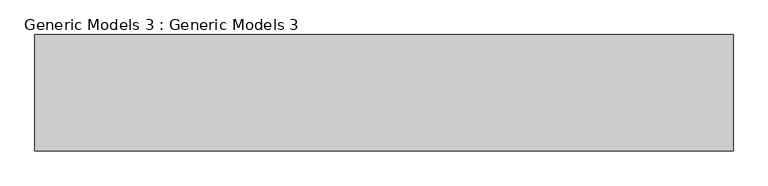
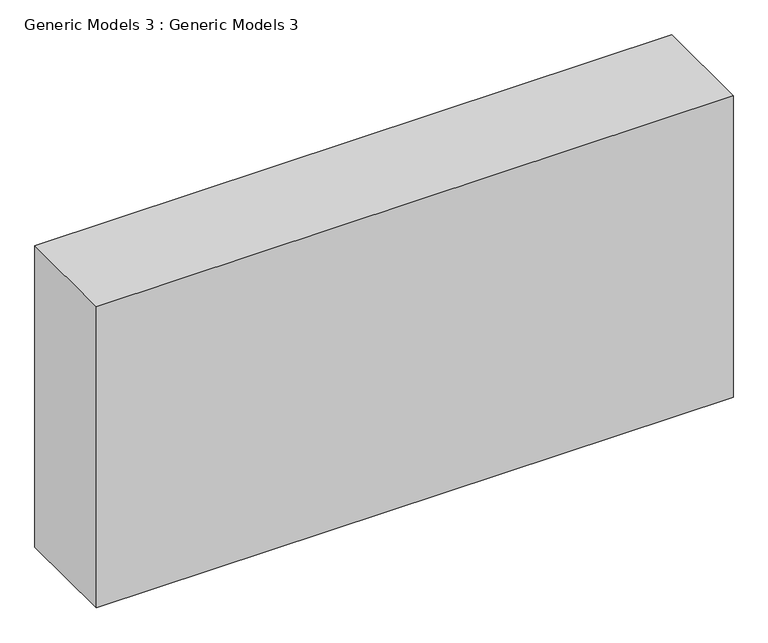
"""IFC4 building model written with IfcOpenShell, lengths in millimetres: proxy geometry, Generic Models 3 : Generic Models 3."""

from ifc_helpers import new_model, si_unit, frame, origin, place, context, project, spatial, polyline, outline, extrude, source, transform, mapped, element, save


def generic_models_3_generic_models_3_5aabad8c(model_context):
    return source(origin(), model_context, "Body", "SweptSolid", [
        extrude(outline(polyline([(-333.0638624, -3729.0064015), (-2161.8638624, -3729.0064015), (-2161.8638624, -3424.2064015), (-333.0638624, -3424.2064015), (-333.0638624, -3729.0064015)])), frame((0.0, 0.0, 9833.369894), z_axis=(0.0, 0.0, 1.0), x_axis=(1.0, 0.0, 0.0)), (0.0, 0.0, 1.0), 914.4),
    ])


if __name__ == "__main__":
    model = new_model("IFC4")
    model_context = context("Model", 3, world=origin())
    ifc_project = project(units=[si_unit("LENGTHUNIT", "METRE", prefix="MILLI")], contexts=[model_context])
    site = spatial("IfcSite", under=ifc_project)
    building = spatial("IfcBuilding", under=site)
    placement = place(None, origin())
    generic_models_3_generic_models_3_shape = generic_models_3_generic_models_3_5aabad8c(model_context)
    element("IfcBuildingElementProxy", 1, Name="Generic Models 3 : Generic Models 3", ObjectType="Generic Models 3 : Generic Models 3", at=placement, inside=building, context=model_context, shape_type="MappedRepresentation", body=[
        mapped(generic_models_3_generic_models_3_shape, transform((0.0, 0.0, 0.0), x_axis=(1.0, 0.0, 0.0), y_axis=(0.0, 1.0, 0.0), z_axis=(0.0, 0.0, 1.0))),
    ])
    save(model, "model.ifc")

# Revit data of these elements
# Element 1 (IfcBuildingElementProxy, "Generic Models 3 : Generic Models 3")
#   Materials on its faces: "Parking Stripe"
# Materials
#   "Parking Stripe": class "Paint", colour RGB 250 250 91, transparency 0, Cost = 0
